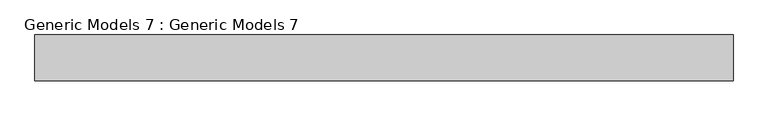
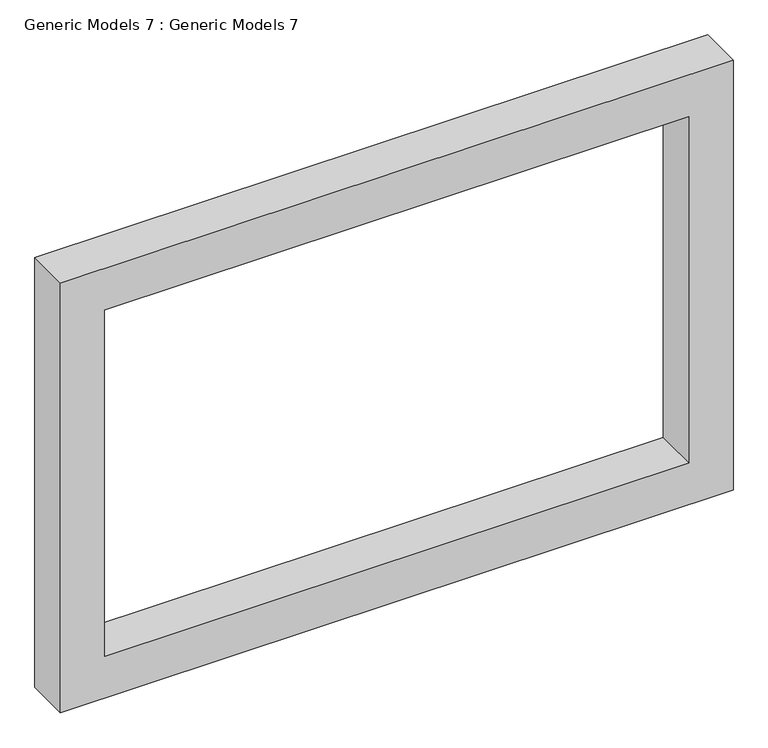
"""IFC4 building model written with IfcOpenShell, lengths in millimetres: proxy geometry, Generic Models 7 : Generic Models 7."""

from ifc_helpers import new_model, si_unit, frame, origin, place, context, project, spatial, polyline, outline, extrude, source, transform, mapped, element, save


def generic_models_7_generic_models_7_0c2edacf(model_context):
    return source(origin(), model_context, "Body", "SweptSolid", [
        extrude(outline(polyline([(2717.2, -3351.3474631), (2717.2, -5666.1474631), (1152.4, -5666.1474631), (1152.4, -3351.3474631), (2717.2, -3351.3474631)]), holes=[polyline([(2564.8, -3503.7474631), (1304.8, -3503.7474631), (1304.8, -5513.7474631), (2564.8, -5513.7474631), (2564.8, -3503.7474631)])]), frame((0.0, -4424.6938352, 0.0), z_axis=(0.0, 1.0, 0.0), x_axis=(0.0, 0.0, 1.0)), (0.0, 0.0, 1.0), 152.4),
    ])


if __name__ == "__main__":
    model = new_model("IFC4")
    model_context = context("Model", 3, world=origin())
    ifc_project = project(units=[si_unit("LENGTHUNIT", "METRE", prefix="MILLI")], contexts=[model_context])
    site = spatial("IfcSite", under=ifc_project)
    building = spatial("IfcBuilding", under=site)
    placement = place(None, origin())
    generic_models_7_generic_models_7_shape = generic_models_7_generic_models_7_0c2edacf(model_context)
    element("IfcBuildingElementProxy", 1, Name="Generic Models 7 : Generic Models 7", ObjectType="Generic Models 7 : Generic Models 7", at=placement, inside=building, context=model_context, shape_type="MappedRepresentation", body=[
        mapped(generic_models_7_generic_models_7_shape, transform((0.0, 0.0, 0.0), x_axis=(1.0, 0.0, 0.0), y_axis=(0.0, 1.0, 0.0), z_axis=(0.0, 0.0, 1.0))),
    ])
    save(model, "model.ifc")

# Revit data of these elements
# Element 1 (IfcBuildingElementProxy, "Generic Models 7 : Generic Models 7")
#   Materials on its faces: "WALL PAINT"
# Materials
#   "WALL PAINT": class "Generic", colour RGB 120 120 120, transparency 0, Cost = 0
